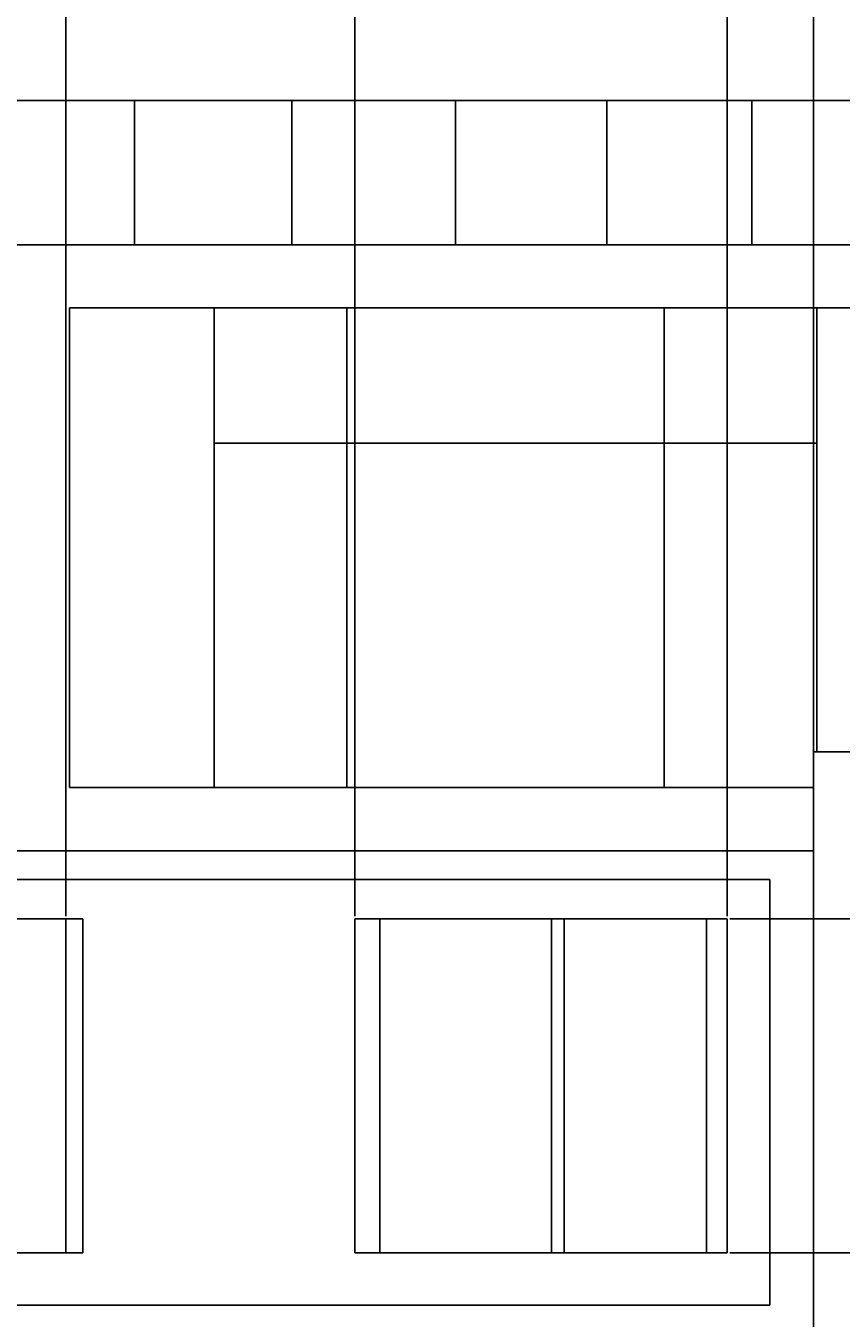
# Model space of a CAD drawing. Units: inches. Extents: x -117 to 121, y -77 to 40.
# Tile 13 of 45: x -64 to -45, y -23 to 7. Entities that reach past the tile are written whole.
import ezdxf

# ---------------------------------------------------------------- set-up
doc = ezdxf.new("R2010")
doc.units = ezdxf.units.IN
doc.header["$MEASUREMENT"] = 0
doc.layers.add('A-ANNO-DIMS', color=2, linetype='Continuous', lineweight=18)
doc.layers.add('A-ELEV', color=7, linetype='Continuous', lineweight=25)
doc.styles.get("Standard").update_dxf_attribs({"font": 'arial.ttf'})
doc.dimstyles.get("Standard").update_dxf_attribs({"dimtxt": 0.18, "dimasz": 0.18, "dimexe": 0.18, "dimexo": 0.0625, "dimgap": 0.09, "dimtad": 0, "dimtih": 1, "dimtoh": 1, "dimdec": 4, "dimzin": 0, "dimdsep": 46, "dimtxsty": 'Standard', "dimcen": 0.09, "dimadec": 0, "dimazin": 0, "dimtfac": 1, "dimtdec": 4, "dimtofl": 0, "dimtmove": 0, "dimatfit": 3, "dimfxl": 1, "dimtolj": 1, "dimtzin": 0, "dimarcsym": 0})

# ---------------------------------------------------------------- blocks, each defined once
blk = doc.blocks.new('*D13')
at = {"layer": 'A-ANNO-DIMS', "color": 0, "lineweight": -2, "transparency": 16777216}
for p, q in [((-2.663, 27.063), (-117.024, 27.063)), ((-116.844, 26.883), (-116.844, -16.974)), ((-116.844, -61.196), (-116.844, -17.338)), ((-106.096, -61.376), (-117.024, -61.376))]:
    blk.add_line(p, q, dxfattribs=at)
at = {"layer": 'A-ANNO-DIMS', "color": 0, "transparency": 16777216}
for points in [[(-116.874, 26.883), (-116.814, 26.883), (-116.844, 27.063)], [(-116.874, -61.196), (-116.814, -61.196), (-116.844, -61.376)]]:
    blk.add_solid(points, dxfattribs=at)
at = {"layer": 'Defpoints', "color": 0, "transparency": 16777216}
for p in [(-2.6, 27.063), (-116.844, -61.376), (-106.034, -61.376)]:
    blk.add_point(p, dxfattribs=at)
at = {"layer": 'A-ANNO-DIMS', "color": 0, "transparency": 16777216, "insert": (-116.844, -17.156), "char_height": 0.18, "attachment_point": 5}
blk.add_mtext('\\A1;88.44', dxfattribs=at)
blk = doc.blocks.new('*D40')
at = {"layer": 'A-ANNO-DIMS', "color": 0, "lineweight": -2, "transparency": 16777216}
for p, q in [((-86.023, -13.677), (-86.023, 38.61)), ((-63.159, -13.677), (-63.159, 38.61)), ((-85.843, 38.43), (-75.056, 38.43)), ((-63.339, 38.43), (-74.126, 38.43))]:
    blk.add_line(p, q, dxfattribs=at)
at = {"layer": 'A-ANNO-DIMS', "color": 0, "transparency": 16777216}
for points in [[(-85.843, 38.46), (-85.843, 38.4), (-86.023, 38.43)], [(-63.339, 38.46), (-63.339, 38.4), (-63.159, 38.43)]]:
    blk.add_solid(points, dxfattribs=at)
at = {"layer": 'Defpoints', "color": 0, "transparency": 16777216}
for p in [(-63.159, 38.43), (-86.023, -13.74), (-63.159, -13.74)]:
    blk.add_point(p, dxfattribs=at)
at = {"layer": 'A-ANNO-DIMS', "color": 0, "transparency": 16777216, "insert": (-74.591, 38.43), "char_height": 0.18, "attachment_point": 5}
blk.add_mtext('\\A1;22.864', dxfattribs=at)
blk = doc.blocks.new('*D41')
at = {"layer": 'A-ANNO-DIMS', "color": 0, "lineweight": -2, "transparency": 16777216}
for p, q in [((-63.159, -13.677), (-63.159, 38.61)), ((-56.33, -13.677), (-56.33, 38.61)), ((-62.979, 38.43), (-60.139, 38.43)), ((-56.51, 38.43), (-59.35, 38.43))]:
    blk.add_line(p, q, dxfattribs=at)
at = {"layer": 'A-ANNO-DIMS', "color": 0, "transparency": 16777216}
for points in [[(-62.979, 38.46), (-62.979, 38.4), (-63.159, 38.43)], [(-56.51, 38.46), (-56.51, 38.4), (-56.33, 38.43)]]:
    blk.add_solid(points, dxfattribs=at)
at = {"layer": 'Defpoints', "color": 0, "transparency": 16777216}
for p in [(-56.33, 38.43), (-63.159, -13.74), (-56.33, -13.74)]:
    blk.add_point(p, dxfattribs=at)
at = {"layer": 'A-ANNO-DIMS', "color": 0, "transparency": 16777216, "insert": (-59.744, 38.43), "char_height": 0.18, "attachment_point": 5}
blk.add_mtext('\\A1;6.829', dxfattribs=at)
blk = doc.blocks.new('*D42')
at = {"layer": 'A-ANNO-DIMS', "color": 0, "lineweight": -2, "transparency": 16777216}
for p, q in [((-56.33, -13.677), (-56.33, 38.61)), ((-47.521, -13.677), (-47.521, 38.61)), ((-56.15, 38.43), (-52.319, 38.43)), ((-47.701, 38.43), (-51.531, 38.43))]:
    blk.add_line(p, q, dxfattribs=at)
at = {"layer": 'A-ANNO-DIMS', "color": 0, "transparency": 16777216}
for points in [[(-56.15, 38.46), (-56.15, 38.4), (-56.33, 38.43)], [(-47.701, 38.46), (-47.701, 38.4), (-47.521, 38.43)]]:
    blk.add_solid(points, dxfattribs=at)
at = {"layer": 'Defpoints', "color": 0, "transparency": 16777216}
for p in [(-47.521, 38.43), (-56.33, -13.74), (-47.521, -13.74)]:
    blk.add_point(p, dxfattribs=at)
at = {"layer": 'A-ANNO-DIMS', "color": 0, "transparency": 16777216, "insert": (-51.925, 38.43), "char_height": 0.18, "attachment_point": 5}
blk.add_mtext('\\A1;8.809', dxfattribs=at)
blk = doc.blocks.new('*D43')
at = {"layer": 'A-ANNO-DIMS', "color": 0, "lineweight": -2, "transparency": 16777216}
for p, q in [((-47.521, -13.677), (-47.521, 38.61)), ((-45.485, -12.071), (-45.485, 38.61)), ((-47.341, 38.43), (-46.898, 38.43)), ((-45.665, 38.43), (-46.108, 38.43))]:
    blk.add_line(p, q, dxfattribs=at)
at = {"layer": 'A-ANNO-DIMS', "color": 0, "transparency": 16777216}
for points in [[(-47.341, 38.46), (-47.341, 38.4), (-47.521, 38.43)], [(-45.665, 38.46), (-45.665, 38.4), (-45.485, 38.43)]]:
    blk.add_solid(points, dxfattribs=at)
at = {"layer": 'Defpoints', "color": 0, "transparency": 16777216}
for p in [(-45.485, 38.43), (-45.485, -12.133), (-47.521, -13.74)]:
    blk.add_point(p, dxfattribs=at)
at = {"layer": 'A-ANNO-DIMS', "color": 0, "transparency": 16777216, "insert": (-46.503, 38.43), "char_height": 0.18, "attachment_point": 5}
blk.add_mtext('\\A1;2.036', dxfattribs=at)
blk = doc.blocks.new('*D50')
at = {"layer": 'A-ANNO-DIMS', "color": 0, "lineweight": -2, "transparency": 16777216}
for p, q in [((-47.458, -13.74), (120.84, -13.74)), ((120.66, -13.92), (120.66, -17.512)), ((120.66, -21.468), (120.66, -17.876)), ((-47.458, -21.648), (120.84, -21.648))]:
    blk.add_line(p, q, dxfattribs=at)
at = {"layer": 'A-ANNO-DIMS', "color": 0, "transparency": 16777216}
for points in [[(120.63, -13.92), (120.69, -13.92), (120.66, -13.74)], [(120.63, -21.468), (120.69, -21.468), (120.66, -21.648)]]:
    blk.add_solid(points, dxfattribs=at)
at = {"layer": 'Defpoints', "color": 0, "transparency": 16777216}
for p in [(-47.521, -13.74), (120.66, -13.74), (-47.521, -21.648)]:
    blk.add_point(p, dxfattribs=at)
at = {"layer": 'A-ANNO-DIMS', "color": 0, "transparency": 16777216, "insert": (120.66, -17.694), "char_height": 0.18, "attachment_point": 5}
blk.add_mtext('\\A1;7.908', dxfattribs=at)

msp = doc.modelspace()

# ---------------------------------------------------------------- linework, layer by layer
at = {"layer": 'A-ELEV'}
for p, q in [((-23.8637, 5.6231), (-74.3507, 5.6231)), ((-61.5403, 2.2073), (-61.5403, 5.6231)), ((-57.8164, 2.2073), (-57.8164, 5.6231)), ((-53.9435, 2.2073), (-53.9435, 5.6231)), ((-50.3685, 2.2073), (-50.3685, 5.6231)), ((-46.9425, 2.2073), (-46.9425, 5.6231)), ((-64.513, 2.2073), (-27.4892, 2.2073)), ((-28.7689, 0.7128), (-63.0775, 0.7128)), ((-63.0775, 0.7128), (-63.0775, -10.6313)), ((-59.6566, 0.7128), (-59.6566, -10.6313)), ((-56.5208, 0.7128), (-56.5208, -10.6313)), ((-49.0139, 0.7128), (-49.0139, -10.6313)), ((-45.403, 0.7128), (-45.403, -9.7904)), ((-59.6566, -2.4907), (-45.403, -2.4907)), ((-45.4848, -12.1334), (-45.4848, -9.7904)), ((-45.4848, -9.7904), (-23.8637, -9.7904)), ((-63.0775, -10.6313), (-45.4848, -10.6313)), ((-64.513, -12.1334), (-45.4848, -12.1334)), ((-45.4848, -12.1334), (-45.4848, -24.6358)), ((-64.513, -12.8131), (-46.5108, -12.8131)), ((-46.5108, -22.8827), (-46.5108, -12.8131)), ((-64.513, -13.74), (-62.763, -13.74)), ((-63.1589, -21.6476), (-63.1589, -13.74)), ((-62.763, -21.6476), (-62.763, -13.74)), ((-56.3295, -21.6476), (-56.3295, -13.74)), ((-56.3295, -13.74), (-47.5206, -13.74)), ((-55.7357, -21.6476), (-55.7357, -13.74)), ((-51.6776, -21.6476), (-51.6776, -13.74)), ((-51.3807, -21.6476), (-51.3807, -13.74)), ((-48.0155, -21.6476), (-48.0155, -13.74)), ((-47.5206, -21.6476), (-47.5206, -13.74)), ((-64.513, -21.6476), (-62.763, -21.6476)), ((-56.3295, -21.6476), (-47.5206, -21.6476)), ((-46.5108, -22.8827), (-93.028, -22.8827))]:
    msp.add_line(p, q, dxfattribs=at)

# ---------------------------------------------------------------- dimensions: what is measured, and where the dimension line sits
at = {"layer": 'A-ANNO-DIMS'}
for base, p1, p2, picture, middle in [((-63.1589, 38.4297), (-86.0225, -13.74), (-63.1589, -13.74), '*D40', (-74.5907, 38.4297)), ((-56.3295, 38.4297), (-63.1589, -13.74), (-56.3295, -13.74), '*D41', (-59.7442, 38.4297)), ((-47.5206, 38.4297), (-56.3295, -13.74), (-47.5206, -13.74), '*D42', (-51.9251, 38.4297)), ((-45.4848, 38.4297), (-47.5206, -13.74), (-45.4848, -12.1334), '*D43', (-46.5027, 38.4297))]:
    dim = msp.add_linear_dim(base=base, p1=p1, p2=p2, dimstyle='Standard', override={"dimdec": 3, "dimlfac": 1, "dimrnd": 0, "dimzin": 0, "dimdsep": 46, "dimlunit": 2}, dxfattribs=at)
    dim.commit()
    dim.dimension.update_dxf_attribs({"geometry": picture, "text_midpoint": middle})
for base, p1, p2, override, picture, middle in [((-116.8438, -61.3756), (-2.6001, 27.0634), (-106.0338, -61.3756), {"dimdec": 2, "dimlfac": 1, "dimrnd": 0, "dimzin": 0, "dimdsep": 46, "dimlunit": 2}, '*D13', (-116.8438, -17.1561)), ((120.6602, -13.74), (-47.5206, -21.6476), (-47.5206, -13.74), {"dimdec": 3, "dimlfac": 1, "dimrnd": 0, "dimzin": 0, "dimdsep": 46, "dimlunit": 2}, '*D50', (120.6602, -17.6938))]:
    dim = msp.add_linear_dim(base=base, p1=p1, p2=p2, angle=90, dimstyle='Standard', override=override, dxfattribs=at)
    dim.commit()
    dim.dimension.update_dxf_attribs({"geometry": picture, "text_midpoint": middle})

doc.saveas('drawing.dxf')
